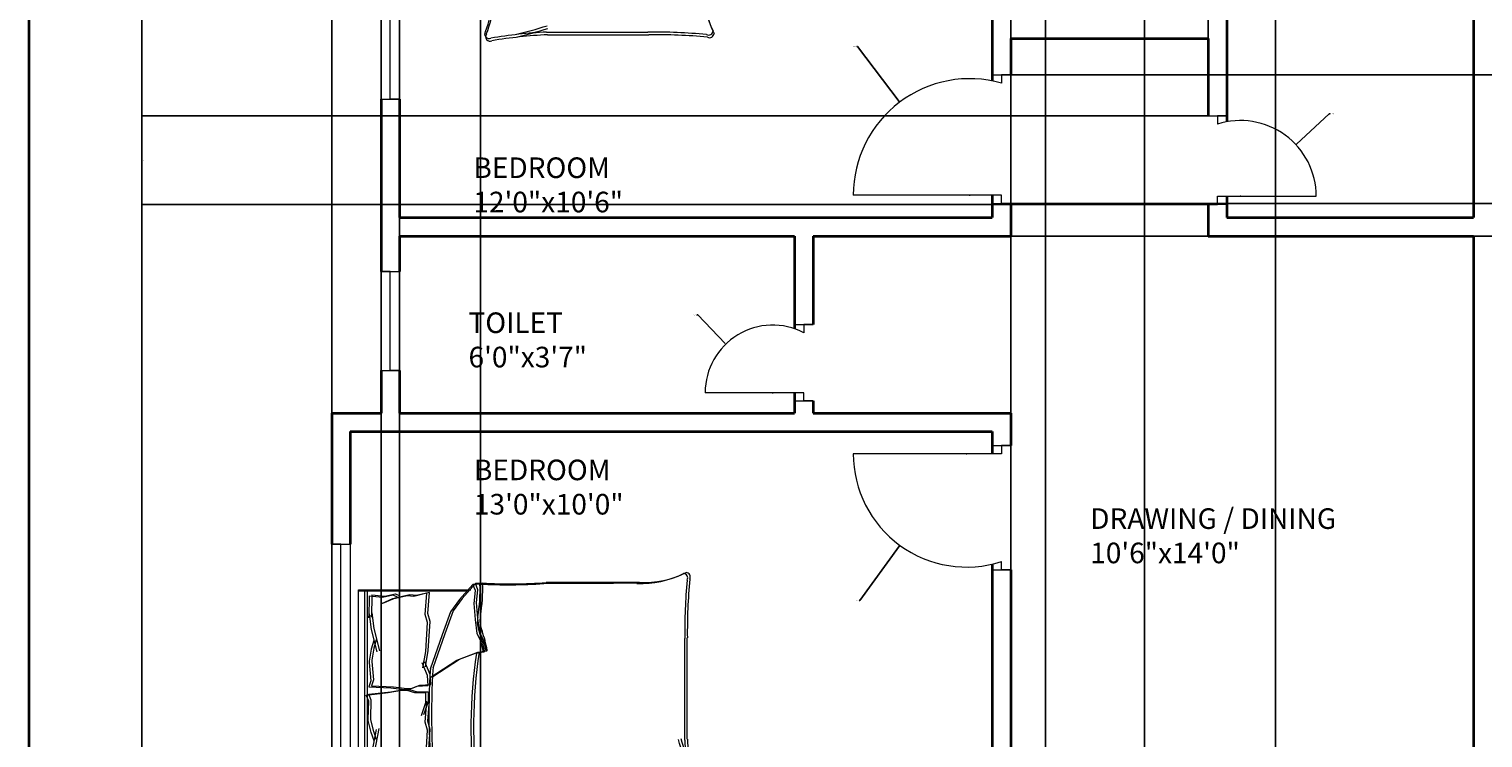
# Model space of a CAD drawing. Units: inches. Extents: x 1937 to 2996, y 1402 to 2323.
# Tile 5 of 10: x 1937 to 2290, y 1944 to 2116. Entities that reach past the tile are written whole.
import ezdxf

# ---------------------------------------------------------------- set-up
doc = ezdxf.new("R2010")
doc.units = ezdxf.units.IN
for name, color, linetype, lineweight in [('A-ANNO-DIMS', 2, 'Continuous', 18), ('A-ANNO-TTLB', 7, 'Continuous', 35), ('A-AREA-IDEN', 7, 'Continuous', 18), ('A-DOOR', 11, 'Continuous', 18), ('A-FURN', 8, 'Continuous', 13), ('A-GLAZ', 141, 'Continuous', 18), ('A-WALL', 7, 'Continuous', 35)]:
    doc.layers.add(name, color=color, linetype=linetype, lineweight=lineweight)
doc.styles.get("Standard").update_dxf_attribs({"font": 'arial.ttf'})
doc.dimstyles.get("Standard").update_dxf_attribs({"dimtxt": 0.18, "dimasz": 0.18, "dimexe": 0.18, "dimexo": 0.0625, "dimgap": 0.09, "dimtad": 0, "dimtih": 1, "dimtoh": 1, "dimdec": 4, "dimzin": 0, "dimdsep": 46, "dimtxsty": 'Standard', "dimcen": 0.09, "dimadec": 0, "dimazin": 0, "dimtfac": 1, "dimtdec": 4, "dimtofl": 0, "dimtmove": 0, "dimatfit": 3, "dimfxl": 1, "dimtolj": 1, "dimtzin": 0, "dimarcsym": 0})

# ---------------------------------------------------------------- blocks, each defined once
blk = doc.blocks.new('BED-DOUBLE')
for p, q in [((-24.01, -18.11), (-24.01, 0)), ((-24.01, -18.11), (-24.01, 0)), ((-24.01, 0), (24.01, 0)), ((23.78, 0), (23.78, -26.61)), ((23.78, 0), (23.78, -26.61)), ((24.01, 0), (24.01, -0.64)), ((-24.01, -1.53), (23.78, -1.53)), ((-24.01, -1.53), (23.78, -1.53)), ((-23.78, -18.75), (-23.78, -0.64)), ((-23.78, -18.75), (-23.78, -0.64)), ((-23.78, -2.17), (24.01, -2.17)), ((-23.78, -2.17), (24.01, -2.17)), ((-23.59, -3.34), (-19.3, -3.01)), ((-23.59, -3.34), (-19.31, -3.01)), ((-23.59, -3.32), (-23.01, -6.5)), ((-23.59, -3.32), (-23.01, -6.5)), ((-19.31, -3.01), (-19.2, -3.03)), ((-19.3, -3.01), (-19.2, -3.03)), ((-19.2, -3.03), (-15.38, -3.32)), ((-19.2, -3.03), (-15.38, -3.32)), ((-15.38, -3.32), (-9.88, -4.33)), ((-15.38, -3.32), (-9.88, -4.33)), ((-12.63, -3.75), (-10.61, -3.03)), ((-12.63, -3.75), (-10.61, -3.03)), ((-10.61, -3.03), (-7.71, -2.3)), ((-10.61, -3.03), (-7.71, -2.3)), ((-10.38, -3.67), (-7.49, -2.94)), ((-10.38, -3.67), (-7.49, -2.94)), ((-7.71, -2.3), (-7.39, -2.3)), ((-7.71, -2.3), (-7.39, -2.3)), ((-7.49, -2.94), (-7.16, -2.94)), ((-7.49, -2.94), (-7.16, -2.94)), ((-7.39, -2.3), (-2.95, -2.45)), ((-7.39, -2.3), (-2.95, -2.45)), ((-7.16, -2.94), (-2.72, -3.09)), ((-7.16, -2.94), (-2.72, -3.09)), ((-2.95, -2.45), (-1.5, -1.87)), ((-2.95, -2.45), (-1.5, -1.87)), ((-2.72, -3.09), (-1.27, -2.51)), ((-2.72, -3.09), (-1.27, -2.51)), ((-1.5, -1.87), (-0.92, -7.22)), ((-1.5, -1.87), (-0.92, -7.22)), ((-1.27, -2.51), (-0.7, -7.86)), ((-1.27, -2.51), (-0.7, -7.86)), ((0.49, -2.49), (0.25, -7.87)), ((0.49, -2.49), (0.25, -7.87)), ((0.72, -3.13), (0.48, -8.51)), ((0.72, -3.13), (0.48, -8.51)), ((1.97, -2.98), (0.49, -2.49)), ((1.97, -2.98), (0.49, -2.49)), ((2.2, -3.62), (0.72, -3.13)), ((2.2, -3.62), (0.72, -3.13)), ((6.4, -2.56), (1.97, -2.98)), ((6.4, -2.56), (1.97, -2.98)), ((6.63, -3.2), (2.2, -3.62)), ((6.63, -3.2), (2.2, -3.62)), ((6.72, -2.54), (6.4, -2.56)), ((6.72, -2.54), (6.4, -2.56)), ((6.95, -3.18), (6.63, -3.2)), ((6.95, -3.18), (6.63, -3.2)), ((9.65, -3.08), (6.72, -2.54)), ((9.65, -3.08), (6.72, -2.54)), ((9.88, -3.72), (6.95, -3.18)), ((9.88, -3.72), (6.95, -3.18)), ((14.43, -3.07), (9.01, -4.42)), ((14.43, -3.07), (9.01, -4.42)), ((11.72, -3.67), (9.65, -3.08)), ((11.72, -3.67), (9.65, -3.08)), ((18.23, -2.54), (14.43, -3.07)), ((18.23, -2.54), (14.43, -3.07)), ((18.46, -3.18), (14.66, -3.71)), ((18.46, -3.18), (14.66, -3.71)), ((22.63, -2.56), (17.23, -2.46)), ((17.23, -2.46), (18.23, -2.54)), ((22.63, -2.56), (17.23, -2.46)), ((17.23, -2.46), (18.23, -2.54)), ((22.86, -3.2), (17.45, -3.1)), ((17.45, -3.1), (18.46, -3.18)), ((22.86, -3.2), (17.45, -3.1)), ((17.45, -3.1), (18.46, -3.18)), ((22.63, -2.56), (22.25, -5.77)), ((22.63, -2.56), (22.25, -5.77)), ((22.86, -3.2), (22.48, -6.41)), ((22.86, -3.2), (22.48, -6.41)), ((24.01, -0.64), (24.01, -27.25)), ((24.01, -0.64), (24.01, -27.25)), ((-23.01, -6.5), (-23.45, -9.1)), ((-23.01, -6.5), (-23.45, -9.1)), ((-23.36, -3.98), (-19.08, -3.65)), ((-23.36, -3.98), (-19.08, -3.65)), ((-23.36, -3.96), (-22.78, -7.14)), ((-23.36, -3.96), (-22.78, -7.14)), ((-22.43, -8.96), (-21.42, -6.21)), ((-22.43, -8.96), (-21.42, -6.21)), ((-22.21, -9.59), (-21.19, -6.85)), ((-22.2, -9.59), (-21.19, -6.85)), ((-19.08, -3.65), (-18.97, -3.67)), ((-19.08, -3.65), (-18.97, -3.67)), ((-18.97, -3.67), (-15.15, -3.96)), ((-18.97, -3.67), (-15.15, -3.96)), ((-15.15, -3.96), (-9.65, -4.97)), ((-15.15, -3.96), (-9.65, -4.97)), ((-12.4, -4.39), (-10.38, -3.67)), ((-12.4, -4.39), (-10.38, -3.67)), ((14.66, -3.71), (9.24, -5.06)), ((14.66, -3.71), (9.24, -5.06)), ((11.94, -4.31), (9.88, -3.72)), ((11.94, -4.31), (9.88, -3.72)), ((21.83, -8.26), (20.64, -5.58)), ((21.82, -8.26), (20.64, -5.58)), ((22.05, -8.9), (20.87, -6.22)), ((22.05, -8.9), (20.87, -6.22)), ((22.25, -5.77), (22.84, -8.34)), ((22.25, -5.77), (22.84, -8.34)), ((22.48, -6.41), (23.07, -8.98)), ((22.48, -6.41), (23.07, -8.98)), ((-23.45, -9.1), (-22.87, -10.11)), ((-23.45, -9.1), (-22.87, -10.11)), ((-22.78, -7.14), (-23.22, -9.74)), ((-22.78, -7.14), (-23.22, -9.74)), ((-23.22, -9.74), (-22.64, -10.75)), ((-23.22, -9.74), (-22.64, -10.75)), ((-23.01, -12.57), (-22.43, -8.96)), ((-23.01, -12.57), (-22.43, -8.96)), ((-22.78, -13.21), (-22.2, -9.59)), ((-22.78, -13.21), (-22.21, -9.59)), ((-0.92, -7.22), (-0.35, -10.4)), ((-0.92, -7.22), (-0.35, -10.4)), ((-0.7, -7.86), (-0.12, -11.04)), ((-0.7, -7.86), (-0.12, -11.04)), ((-0.35, -10.4), (-0.35, -11.7)), ((-0.35, -10.4), (-0.35, -11.7)), ((0.25, -7.87), (-0.13, -11.08)), ((0.25, -7.87), (-0.13, -11.08)), ((0.48, -8.51), (0.1, -11.72)), ((0.48, -8.51), (0.1, -11.72)), ((22.63, -11.83), (21.82, -8.26)), ((22.63, -11.83), (21.83, -8.26)), ((22.86, -12.47), (22.05, -8.9)), ((22.86, -12.47), (22.05, -8.9)), ((22.84, -8.34), (22.33, -9.38)), ((22.84, -8.34), (22.33, -9.38)), ((23.07, -8.98), (22.56, -10.02)), ((23.07, -8.98), (22.56, -10.02)), ((-22.72, -14.16), (-23.01, -12.57)), ((-22.72, -14.16), (-23.01, -12.57)), ((-22.49, -14.8), (-22.78, -13.21)), ((-22.49, -14.8), (-22.78, -13.21)), ((-0.35, -11.7), (-0.92, -13.58)), ((-0.35, -11.7), (-0.92, -13.58)), ((-0.92, -13.58), (-0.92, -16.26)), ((-0.92, -13.58), (-0.92, -16.26)), ((-0.12, -12.34), (-0.7, -14.22)), ((-0.12, -12.34), (-0.7, -14.22)), ((-0.13, -11.08), (-0.05, -12.38)), ((-0.13, -11.08), (-0.05, -12.38)), ((-0.12, -11.04), (-0.12, -12.34)), ((-0.12, -11.04), (-0.12, -12.34)), ((-0.05, -12.38), (0.65, -14.22)), ((-0.05, -12.38), (0.65, -14.22)), ((0.1, -11.72), (0.18, -13.02)), ((0.1, -11.72), (0.18, -13.02)), ((0.18, -13.02), (0.87, -14.86)), ((0.18, -13.02), (0.87, -14.86)), ((22.44, -13.43), (22.63, -11.83)), ((22.44, -13.43), (22.63, -11.83)), ((23.21, -16.57), (22.44, -13.43)), ((23.21, -16.57), (22.44, -13.43)), ((22.67, -14.07), (22.86, -12.47)), ((22.67, -14.07), (22.86, -12.47)), ((23.44, -17.21), (22.67, -14.07)), ((23.44, -17.21), (22.67, -14.07)), ((-23.3, -17.34), (-22.72, -14.16)), ((-23.3, -17.34), (-22.72, -14.16)), ((-18.2, -16.62), (-23.3, -17.34)), ((-18.2, -16.62), (-23.3, -17.34)), ((-23.07, -17.98), (-22.49, -14.8)), ((-23.07, -17.98), (-22.49, -14.8)), ((-17.98, -17.26), (-23.07, -17.98)), ((-17.98, -17.26), (-23.07, -17.98)), ((-21.1, -15.63), (-17.07, -16.3)), ((-21.1, -15.63), (-17.07, -16.3)), ((-20.87, -16.27), (-16.84, -16.93)), ((-20.87, -16.27), (-16.84, -16.93)), ((-17.07, -16.3), (-18.2, -16.62)), ((-17.07, -16.3), (-18.2, -16.62)), ((-16.84, -16.93), (-17.98, -17.26)), ((-16.84, -16.93), (-17.98, -17.26)), ((-17.07, -16.3), (-10.06, -16.73)), ((-17.07, -16.3), (-10.06, -16.73)), ((-16.84, -16.93), (-9.83, -17.37)), ((-16.84, -16.93), (-9.83, -17.37)), ((-10.06, -16.73), (-8.1, -16.17)), ((-10.06, -16.73), (-8.1, -16.17)), ((-9.83, -17.37), (-7.87, -16.81)), ((-9.83, -17.37), (-7.87, -16.81)), ((-8.1, -16.17), (-2.97, -16.57)), ((-8.1, -16.17), (-2.97, -16.57)), ((-7.87, -16.81), (-2.74, -17.21)), ((-7.87, -16.81), (-2.74, -17.21)), ((-3.38, -16.26), (-6.53, -15.17)), ((-3.38, -16.26), (-6.53, -15.17)), ((-3.15, -16.9), (-6.3, -15.81)), ((-3.15, -16.9), (-6.3, -15.81)), ((-0.92, -16.26), (-3.38, -16.26)), ((-0.92, -16.26), (-3.38, -16.26)), ((-0.7, -16.9), (-3.15, -16.9)), ((-0.7, -16.9), (-3.15, -16.9)), ((-0.7, -14.22), (-0.7, -16.9)), ((-0.7, -14.22), (-0.7, -16.9)), ((0.65, -14.22), (0.81, -16.89)), ((0.65, -14.22), (0.81, -16.89)), ((0.81, -16.89), (3.27, -16.74)), ((0.81, -16.89), (3.27, -16.74)), ((0.87, -14.86), (1.04, -17.53)), ((0.87, -14.86), (1.04, -17.53)), ((1.04, -17.53), (3.49, -17.38)), ((1.04, -17.53), (3.49, -17.38)), ((2.77, -17.38), (6.97, -23.88)), ((2.77, -17.38), (6.96, -23.88)), ((3.27, -16.74), (6.34, -15.45)), ((3.27, -16.74), (6.34, -15.45)), ((3.49, -17.38), (6.56, -16.09)), ((3.49, -17.38), (6.56, -16.09)), ((13.16, -20.32), (4.82, -17.38)), ((13.16, -20.32), (4.82, -17.38)), ((5.08, -15.63), (9.11, -16.3)), ((5.08, -15.63), (9.11, -16.3)), ((5.31, -16.27), (9.34, -16.93)), ((5.31, -16.27), (9.34, -16.93)), ((9.11, -16.3), (16.12, -16.73)), ((9.11, -16.3), (16.12, -16.73)), ((9.34, -16.93), (16.35, -17.37)), ((9.34, -16.93), (16.35, -17.37)), ((16.12, -16.73), (18.08, -16.17)), ((16.12, -16.73), (18.08, -16.17)), ((16.35, -17.37), (18.31, -16.81)), ((16.35, -17.37), (18.31, -16.81)), ((18.08, -16.17), (23.21, -16.57)), ((18.08, -16.17), (23.21, -16.57)), ((18.31, -16.81), (23.44, -17.21)), ((18.31, -16.81), (23.44, -17.21)), ((3, -18.02), (7.19, -24.52)), ((3, -18.02), (7.19, -24.52)), ((13.39, -20.96), (5.05, -18.02)), ((13.39, -20.96), (5.05, -18.02)), ((18.74, -22.33), (13.16, -20.32)), ((18.74, -22.33), (13.16, -20.32)), ((18.96, -22.97), (13.39, -20.96)), ((18.96, -22.97), (13.39, -20.96)), ((6.96, -23.88), (8.67, -28.37)), ((6.97, -23.88), (8.67, -28.37)), ((7.19, -24.52), (8.9, -29)), ((7.19, -24.52), (8.9, -29)), ((21.68, -24.5), (18.74, -22.33)), ((21.68, -24.5), (18.74, -22.33)), ((21.91, -25.13), (18.96, -22.97)), ((21.91, -25.13), (18.96, -22.97)), ((25.38, -27.75), (21.68, -24.5)), ((25.38, -27.75), (21.68, -24.5)), ((16.88, -28.37), (20.75, -28.06)), ((16.88, -28.37), (20.75, -28.06)), ((20.75, -28.06), (23.85, -28.37)), ((20.75, -28.06), (23.85, -28.37)), ((25.61, -28.39), (21.91, -25.13)), ((25.61, -28.39), (21.91, -25.13)), ((23.85, -28.37), (25.38, -27.75)), ((23.85, -28.37), (25.38, -27.75)), ((25.46, -29.49), (25.38, -27.75, 3.87)), ((25.46, -29.49), (25.38, -27.75, 3.87)), ((8.67, -28.37), (8.98, -30.38)), ((8.67, -28.37), (8.98, -30.38)), ((8.9, -29), (9.21, -31.02)), ((8.9, -29), (9.21, -31.02)), ((8.98, -30.38), (11.46, -29.76)), ((8.98, -30.38), (11.46, -29.76)), ((9.21, -31.02), (11.68, -30.4)), ((9.21, -31.02), (11.68, -30.4)), ((11.46, -29.76), (13.47, -28.83)), ((11.46, -29.76), (13.47, -28.83)), ((11.68, -30.4), (13.7, -29.47)), ((11.68, -30.4), (13.7, -29.47)), ((13.47, -28.83), (16.88, -28.37)), ((13.47, -28.83), (16.88, -28.37)), ((13.7, -29.47), (17.11, -29)), ((13.7, -29.47), (17.1, -29)), ((17.1, -29), (20.98, -28.69)), ((17.11, -29), (20.98, -28.69)), ((20.98, -28.69), (24.07, -29)), ((20.98, -28.69), (24.07, -29)), ((24.07, -29), (25.61, -28.39)), ((24.07, -29), (25.61, -28.39)), ((25.69, -30.13), (25.61, -28.39, 3.87)), ((25.69, -30.13), (25.61, -28.39, 3.87)), ((-12.42, -79.25), (12.19, -79.25)), ((-12.42, -79.25), (12.19, -79.25)), ((-12.19, -79.88), (12.42, -79.88)), ((-12.19, -79.88), (12.42, -79.88))]:
    blk.add_line(p, q)
for centre, radius, start, end in [((-6.13, -182.05), 164.97, 86.0865, 96.7821), ((-6.13, -182.05), 164.97, 86.0865, 96.7821), ((57.68, -20.1), 83.31, 178.7218, 185.604), ((57.68, -20.1), 83.31, 178.7218, 185.604), ((57.91, -20.74), 83.31, 178.7218, 185.604), ((57.91, -20.74), 83.31, 178.7218, 185.604), ((-5.9, -182.69), 164.97, 86.0865, 96.7821), ((-5.9, -182.69), 164.97, 86.0865, 96.7821), ((-9.73, -156.32), 129.02, 81.7845, 96.9006), ((-9.73, -156.32), 129.02, 81.7845, 96.9006), ((-9.5, -156.96), 129.02, 81.7845, 96.9006), ((-9.5, -156.96), 129.02, 81.7845, 96.9006), ((-194.79, -31.17), 170.11, 358.4762, 1.0082), ((-194.79, -31.17), 170.11, 358.4762, 1.0082), ((-194.56, -31.81), 170.11, 358.4762, 1.0082), ((-194.56, -31.81), 170.11, 358.4762, 1.0082), ((9.15, -30.44), 0.185, 160.2464, 271.1377), ((9.15, -30.44), 0.185, 160.2464, 271.1377), ((3.67, -1.48), 29.65, 280.6617, 289.8806), ((3.67, -1.48), 29.65, 280.6617, 289.8806), ((9.38, -31.08), 0.185, 160.2464, 271.1377), ((9.38, -31.08), 0.185, 160.2464, 271.1377), ((3.9, -2.12), 29.65, 280.6617, 289.8806), ((3.9, -2.12), 29.65, 280.6617, 289.8806), ((16.26, -35.07), 6.22, 78.6608, 113.7384), ((16.26, -35.07), 6.22, 78.6608, 113.7384), ((16.49, -35.71), 6.22, 78.6608, 113.7384), ((16.49, -35.71), 6.22, 78.6608, 113.7384), ((23.84, 6.66), 36.18, 259.8763, 272.5657), ((23.84, 6.66), 36.18, 259.8763, 272.5657), ((24.07, 6.02), 36.18, 259.8763, 272.5657), ((24.07, 6.02), 36.18, 259.8763, 272.5657), ((154.78, -36.32), 129.5, 176.9791, 183.8365), ((154.78, -36.32), 129.5, 176.9791, 183.8365), ((155.01, -36.95), 129.5, 176.9791, 183.8365), ((155.01, -36.95), 129.5, 176.9791, 183.8365), ((457.34, -50.61), 482.31, 178.2277, 181.7185), ((457.34, -50.61), 482.31, 178.2277, 181.7185), ((457.57, -51.25), 482.31, 178.2277, 181.7185), ((457.57, -51.25), 482.31, 178.2277, 181.7185), ((-4536.23, -67.82), 4561.86, 0.00217, 0.28689), ((-4536.23, -67.82), 4561.86, 0.00217, 0.28689), ((-4536, -68.46), 4561.86, 0.00217, 0.28689), ((-4536, -68.46), 4561.86, 0.00217, 0.28689), ((-54.38, -64.52), 29.63, 346.0648, 358.9113), ((-54.38, -64.52), 29.63, 346.0648, 358.9113), ((-54.16, -65.15), 29.63, 346.0648, 358.9113), ((-54.16, -65.15), 29.63, 346.0648, 358.9113), ((48.67, -68.67), 23.07, 177.4714, 206.4681), ((48.67, -68.67), 23.07, 177.4714, 206.4681), ((48.9, -69.31), 23.07, 177.4714, 206.4681), ((48.9, -69.31), 23.07, 177.4714, 206.4681), ((-49.14, -70.28), 23.56, 337.9751, 356.652), ((-49.14, -70.28), 23.56, 337.9751, 356.652), ((-48.92, -70.91), 23.56, 337.9751, 356.652), ((-48.92, -70.91), 23.56, 337.9751, 356.652), ((-44.71, 23.71), 106.46, 283.3832, 287.7053), ((-44.71, 23.71), 106.46, 283.3832, 287.7053), ((-26.4, -79.72), 1.09, 146.1736, 293.4781), ((-26.4, -79.72), 1.09, 146.1736, 293.4781), ((-26.17, -80.36), 1.09, 146.1736, 293.4781), ((-26.17, -80.36), 1.09, 146.1736, 293.4781), ((-6.06, -200.84), 121.76, 92.9958, 99.4091), ((-6.06, -200.84), 121.76, 92.9958, 99.4091), ((-5.83, -201.48), 121.76, 92.9958, 99.4091), ((-5.83, -201.48), 121.76, 92.9958, 99.4091), ((-44.48, 23.07), 106.46, 283.3832, 287.7053), ((-44.48, 23.07), 106.46, 283.3832, 287.7053), ((13.67, -212.28), 133.04, 84.4998, 90.6351), ((13.67, -212.28), 133.04, 84.4998, 90.6351), ((13.9, -212.92), 133.04, 84.4998, 90.6351), ((13.9, -212.92), 133.04, 84.4998, 90.6351), ((26.93, -78.87), 1.1, 242.6588, 356.02), ((26.93, -78.87), 1.1, 242.6588, 356.02), ((27.15, -79.51), 1.1, 242.6588, 356.02), ((27.15, -79.51), 1.1, 242.6588, 356.02)]:
    blk.add_arc(centre, radius, start, end)
blk = doc.blocks.new('WINDOW-60IN')
for p, q in [((0, 2.25), (0, -2.25)), ((0, 2.25), (60, 2.25)), ((0, -2.25), (0, 0)), ((0, 0), (60, 0)), ((60, 0), (60, 2.25)), ((60, 2.25), (60, -2.25)), ((60, -2.25), (0, -2.25))]:
    blk.add_line(p, q)
blk = doc.blocks.new('WINDOW-24IN')
for p, q in [((0, -2.25), (0, 2.25)), ((0, 2.25), (0, 0)), ((24, 2.25), (0, 2.25)), ((0, 0), (24, 0)), ((24, -2.25), (24, 2.25)), ((24, 0), (24, -2.25)), ((0, -2.25), (24, -2.25))]:
    blk.add_line(p, q)
blk = doc.blocks.new('*D24')
at = {"layer": 'A-ANNO-DIMS', "color": 0, "lineweight": -2, "transparency": 16777216}
for p, q in [((2022.58, 2236.81), (1964.32, 2236.81)), ((1964.5, 2236.63), (1964.5, 1896.24)), ((1964.5, 1555.49), (1964.5, 1895.87)), ((2022.58, 1555.31), (1964.32, 1555.31))]:
    blk.add_line(p, q, dxfattribs=at)
at = {"layer": 'A-ANNO-DIMS', "color": 0, "transparency": 16777216}
for points in [[(1964.47, 2236.63), (1964.53, 2236.63), (1964.5, 2236.81)], [(1964.47, 1555.49), (1964.53, 1555.49), (1964.5, 1555.31)]]:
    blk.add_solid(points, dxfattribs=at)
at = {"layer": 'Defpoints', "color": 0, "transparency": 16777216}
for p in [(1964.5, 2236.81), (2022.65, 2236.81), (2022.65, 1555.31)]:
    blk.add_point(p, dxfattribs=at)
at = {"layer": 'A-ANNO-DIMS', "color": 0, "transparency": 16777216, "insert": (1964.5, 1896.06), "char_height": 0.18, "attachment_point": 5}
blk.add_mtext('\\A1;681.5', dxfattribs=at)
blk = doc.blocks.new('*D44')
at = {"layer": 'A-ANNO-DIMS', "color": 0, "lineweight": -2, "transparency": 16777216}
for p, q in [((2010.65, 1769.37), (2010.65, 2283.14)), ((2010.83, 2282.96), (2016.44, 2282.96)), ((2022.47, 2282.96), (2016.86, 2282.96)), ((2022.65, 1769.37), (2022.65, 2283.14))]:
    blk.add_line(p, q, dxfattribs=at)
at = {"layer": 'A-ANNO-DIMS', "color": 0, "transparency": 16777216}
for points in [[(2010.83, 2282.99), (2010.83, 2282.93), (2010.65, 2282.96)], [(2022.47, 2282.99), (2022.47, 2282.93), (2022.65, 2282.96)]]:
    blk.add_solid(points, dxfattribs=at)
at = {"layer": 'Defpoints', "color": 0, "transparency": 16777216}
for p in [(2022.65, 2282.96), (2010.65, 1769.31), (2022.65, 1769.31)]:
    blk.add_point(p, dxfattribs=at)
at = {"layer": 'A-ANNO-DIMS', "color": 0, "transparency": 16777216, "insert": (2016.65, 2282.96), "char_height": 0.18, "attachment_point": 5}
blk.add_mtext('\\A1;12', dxfattribs=at)
blk = doc.blocks.new('*D46')
at = {"layer": 'A-ANNO-DIMS', "color": 0, "lineweight": -2, "transparency": 16777216}
for p, q in [((2027.15, 1591.37), (2027.15, 2283.14)), ((2027.33, 2282.96), (2036.53, 2282.96)), ((2046.64, 2282.96), (2037.44, 2282.96)), ((2046.82, 1591.37), (2046.82, 2283.14))]:
    blk.add_line(p, q, dxfattribs=at)
at = {"layer": 'A-ANNO-DIMS', "color": 0, "transparency": 16777216}
for points in [[(2027.33, 2282.99), (2027.33, 2282.93), (2027.15, 2282.96)], [(2046.64, 2282.99), (2046.64, 2282.93), (2046.82, 2282.96)]]:
    blk.add_solid(points, dxfattribs=at)
at = {"layer": 'Defpoints', "color": 0, "transparency": 16777216}
for p in [(2046.82, 2282.96), (2027.15, 1591.31), (2046.82, 1591.31)]:
    blk.add_point(p, dxfattribs=at)
at = {"layer": 'A-ANNO-DIMS', "color": 0, "transparency": 16777216, "insert": (2036.99, 2282.96), "char_height": 0.18, "attachment_point": 5}
blk.add_mtext('\\A1;19.678', dxfattribs=at)
blk = doc.blocks.new('*D47')
at = {"layer": 'A-ANNO-DIMS', "color": 0, "lineweight": -2, "transparency": 16777216}
for p, q in [((2175.65, 1591.37), (2175.65, 2283.14)), ((2175.83, 2282.96), (2179.52, 2282.96)), ((2183.96, 2282.96), (2180.27, 2282.96)), ((2184.14, 1591.37), (2184.14, 2283.14))]:
    blk.add_line(p, q, dxfattribs=at)
at = {"layer": 'A-ANNO-DIMS', "color": 0, "transparency": 16777216}
for points in [[(2175.83, 2282.99), (2175.83, 2282.93), (2175.65, 2282.96)], [(2183.96, 2282.99), (2183.96, 2282.93), (2184.14, 2282.96)]]:
    blk.add_solid(points, dxfattribs=at)
at = {"layer": 'Defpoints', "color": 0, "transparency": 16777216}
for p in [(2184.14, 2282.96), (2175.65, 1591.31), (2184.14, 1591.31)]:
    blk.add_point(p, dxfattribs=at)
at = {"layer": 'A-ANNO-DIMS', "color": 0, "transparency": 16777216, "insert": (2179.89, 2282.96), "char_height": 0.18, "attachment_point": 5}
blk.add_mtext('\\A1;8.491', dxfattribs=at)
blk = doc.blocks.new('*D48')
at = {"layer": 'A-ANNO-DIMS', "color": 0, "lineweight": -2, "transparency": 16777216}
for p, q in [((2208.14, 1591.37), (2208.14, 2283.14)), ((2208.32, 2282.96), (2223.66, 2282.96)), ((2239.78, 2282.96), (2224.44, 2282.96)), ((2239.96, 1591.37), (2239.96, 2283.14))]:
    blk.add_line(p, q, dxfattribs=at)
at = {"layer": 'A-ANNO-DIMS', "color": 0, "transparency": 16777216}
for points in [[(2208.32, 2282.99), (2208.32, 2282.93), (2208.14, 2282.96)], [(2239.78, 2282.99), (2239.78, 2282.93), (2239.96, 2282.96)]]:
    blk.add_solid(points, dxfattribs=at)
at = {"layer": 'Defpoints', "color": 0, "transparency": 16777216}
for p in [(2239.96, 2282.96), (2208.14, 1591.31), (2239.96, 1591.31)]:
    blk.add_point(p, dxfattribs=at)
at = {"layer": 'A-ANNO-DIMS', "color": 0, "transparency": 16777216, "insert": (2224.05, 2282.96), "char_height": 0.18, "attachment_point": 5}
blk.add_mtext('\\A1;31.82', dxfattribs=at)
blk = doc.blocks.new('*D49')
at = {"layer": 'A-ANNO-DIMS', "color": 0, "lineweight": -2, "transparency": 16777216}
for p, q in [((2223.65, 2095.03), (2223.65, 2283.14)), ((2223.83, 2282.96), (2225.64, 2282.96)), ((2227.97, 2282.96), (2226.16, 2282.96)), ((2228.15, 2095.03), (2228.15, 2283.14))]:
    blk.add_line(p, q, dxfattribs=at)
at = {"layer": 'A-ANNO-DIMS', "color": 0, "transparency": 16777216}
for points in [[(2223.83, 2282.99), (2223.83, 2282.93), (2223.65, 2282.96)], [(2227.97, 2282.99), (2227.97, 2282.93), (2228.15, 2282.96)]]:
    blk.add_solid(points, dxfattribs=at)
at = {"layer": 'Defpoints', "color": 0, "transparency": 16777216}
for p in [(2228.15, 2282.96), (2223.65, 2094.97), (2228.15, 2094.97)]:
    blk.add_point(p, dxfattribs=at)
at = {"layer": 'A-ANNO-DIMS', "color": 0, "transparency": 16777216, "insert": (2225.9, 2282.96), "char_height": 0.18, "attachment_point": 5}
blk.add_mtext('\\A1;4.5', dxfattribs=at)
blk = doc.blocks.new('*D51')
at = {"layer": 'A-ANNO-DIMS', "color": 0, "lineweight": -2, "transparency": 16777216}
for p, q in [((2175.71, 2073.74), (2970.48, 2073.74)), ((2970.3, 2073.56), (2970.3, 2069.95)), ((2970.3, 2065.99), (2970.3, 2069.59)), ((2175.71, 2065.81), (2970.48, 2065.81))]:
    blk.add_line(p, q, dxfattribs=at)
at = {"layer": 'A-ANNO-DIMS', "color": 0, "transparency": 16777216}
for points in [[(2970.27, 2073.56), (2970.33, 2073.56), (2970.3, 2073.74)], [(2970.27, 2065.99), (2970.33, 2065.99), (2970.3, 2065.81)]]:
    blk.add_solid(points, dxfattribs=at)
at = {"layer": 'Defpoints', "color": 0, "transparency": 16777216}
for p in [(2175.65, 2073.74), (2970.3, 2073.74), (2175.65, 2065.81)]:
    blk.add_point(p, dxfattribs=at)
at = {"layer": 'A-ANNO-DIMS', "color": 0, "transparency": 16777216, "insert": (2970.3, 2069.77), "char_height": 0.18, "attachment_point": 5}
blk.add_mtext('\\A1;7.931', dxfattribs=at)
blk = doc.blocks.new('*D52')
at = {"layer": 'A-ANNO-DIMS', "color": 0, "lineweight": -2, "transparency": 16777216}
for p, q in [((2175.71, 2104.94), (2970.48, 2104.94)), ((2970.3, 2104.76), (2970.3, 2089.52)), ((2970.3, 2073.92), (2970.3, 2089.16)), ((2175.71, 2073.74), (2970.48, 2073.74))]:
    blk.add_line(p, q, dxfattribs=at)
at = {"layer": 'A-ANNO-DIMS', "color": 0, "transparency": 16777216}
for points in [[(2970.27, 2104.76), (2970.33, 2104.76), (2970.3, 2104.94)], [(2970.27, 2073.92), (2970.33, 2073.92), (2970.3, 2073.74)]]:
    blk.add_solid(points, dxfattribs=at)
at = {"layer": 'Defpoints', "color": 0, "transparency": 16777216}
for p in [(2175.65, 2104.94), (2970.3, 2104.94), (2175.65, 2073.74)]:
    blk.add_point(p, dxfattribs=at)
at = {"layer": 'A-ANNO-DIMS', "color": 0, "transparency": 16777216, "insert": (2970.3, 2089.34), "char_height": 0.18, "attachment_point": 5}
blk.add_mtext('\\A1;31.204', dxfattribs=at)
blk = doc.blocks.new('*D54')
at = {"layer": 'A-ANNO-DIMS', "color": 0, "lineweight": -2, "transparency": 16777216}
for p, q in [((2223.58, 2094.97), (1964.32, 2094.97)), ((1964.5, 2094.79), (1964.5, 2084.39)), ((1964.5, 2073.63), (1964.5, 2084.03)), ((2223.58, 2073.45), (1964.32, 2073.45))]:
    blk.add_line(p, q, dxfattribs=at)
at = {"layer": 'A-ANNO-DIMS', "color": 0, "transparency": 16777216}
for points in [[(1964.47, 2094.79), (1964.53, 2094.79), (1964.5, 2094.97)], [(1964.47, 2073.63), (1964.53, 2073.63), (1964.5, 2073.45)]]:
    blk.add_solid(points, dxfattribs=at)
at = {"layer": 'Defpoints', "color": 0, "transparency": 16777216}
for p in [(1964.5, 2094.97), (2223.65, 2094.97), (2223.65, 2073.45)]:
    blk.add_point(p, dxfattribs=at)
at = {"layer": 'A-ANNO-DIMS', "color": 0, "transparency": 16777216, "insert": (1964.5, 2084.21), "char_height": 0.18, "attachment_point": 5}
blk.add_mtext('\\A1;21.518', dxfattribs=at)
blk = doc.blocks.new('*D66')
at = {"layer": 'A-ANNO-DIMS', "color": 0, "lineweight": -2, "transparency": 16777216}
for p, q in [((2138.22, 2111.84), (2138.4, 2111.84)), ((2138.4, 2111.84), (2148.52, 2098.44)), ((2165.59, 2075.74), (2165.77, 2075.74)), ((2165.68, 2075.65), (2165.68, 2075.83))]:
    blk.add_line(p, q, dxfattribs=at)
at = {"layer": 'A-ANNO-DIMS', "color": 0, "transparency": 16777216}
blk.add_solid([(2148.54, 2098.46), (2148.49, 2098.42), (2148.63, 2098.3)], dxfattribs=at)
at = {"layer": 'Defpoints', "color": 0, "transparency": 16777216}
for p in [(2148.63, 2098.3), (2165.68, 2075.74)]:
    blk.add_point(p, dxfattribs=at)
at = {"layer": 'A-ANNO-DIMS', "color": 0, "transparency": 16777216, "insert": (2137.74, 2111.84), "char_height": 0.18, "attachment_point": 5}
blk.add_mtext('\\A1;R28.28', dxfattribs=at)
blk = doc.blocks.new('*D68')
at = {"layer": 'A-ANNO-DIMS', "color": 0, "lineweight": -2, "transparency": 16777216}
for p, q in [((2164.84, 2012.95), (2165.02, 2012.95)), ((2164.93, 2012.86), (2164.93, 2013.04)), ((2139.01, 1977.33), (2148.62, 1990.55)), ((2138.83, 1977.33), (2139.01, 1977.33))]:
    blk.add_line(p, q, dxfattribs=at)
at = {"layer": 'A-ANNO-DIMS', "color": 0, "transparency": 16777216}
blk.add_solid([(2148.6, 1990.56), (2148.65, 1990.53), (2148.73, 1990.69)], dxfattribs=at)
at = {"layer": 'Defpoints', "color": 0, "transparency": 16777216}
for p in [(2164.93, 2012.95), (2148.73, 1990.69)]:
    blk.add_point(p, dxfattribs=at)
at = {"layer": 'A-ANNO-DIMS', "color": 0, "transparency": 16777216, "insert": (2138.35, 1977.33), "char_height": 0.18, "attachment_point": 5}
blk.add_mtext('\\A1;R27.53', dxfattribs=at)
blk = doc.blocks.new('*D74')
at = {"layer": 'A-ANNO-DIMS', "color": 0, "lineweight": -2, "transparency": 16777216}
for p, q in [((2253.06, 2095.49), (2245.11, 2088.1)), ((2253.24, 2095.49), (2253.06, 2095.49)), ((2231.41, 2075.45), (2231.59, 2075.45)), ((2231.5, 2075.36), (2231.5, 2075.54))]:
    blk.add_line(p, q, dxfattribs=at)
at = {"layer": 'A-ANNO-DIMS', "color": 0, "transparency": 16777216}
blk.add_solid([(2245.09, 2088.12), (2245.13, 2088.08), (2244.97, 2087.98)], dxfattribs=at)
at = {"layer": 'Defpoints', "color": 0, "transparency": 16777216}
for p in [(2244.97, 2087.98), (2231.5, 2075.45)]:
    blk.add_point(p, dxfattribs=at)
at = {"layer": 'A-ANNO-DIMS', "color": 0, "transparency": 16777216, "insert": (2253.79, 2095.49), "char_height": 0.18, "attachment_point": 5}
blk.add_mtext('\\A1;R18.393', dxfattribs=at)
blk = doc.blocks.new('*D75')
at = {"layer": 'A-ANNO-DIMS', "color": 0, "lineweight": -2, "transparency": 16777216}
for p, q in [((2099.4, 2046.66), (2099.58, 2046.66)), ((2099.58, 2046.66), (2106.29, 2039.7)), ((2117.72, 2027.76), (2117.9, 2027.76)), ((2117.81, 2027.67), (2117.81, 2027.85))]:
    blk.add_line(p, q, dxfattribs=at)
at = {"layer": 'A-ANNO-DIMS', "color": 0, "transparency": 16777216}
blk.add_solid([(2106.31, 2039.72), (2106.27, 2039.68), (2106.42, 2039.57)], dxfattribs=at)
at = {"layer": 'Defpoints', "color": 0, "transparency": 16777216}
for p in [(2106.42, 2039.57), (2117.81, 2027.76)]:
    blk.add_point(p, dxfattribs=at)
at = {"layer": 'A-ANNO-DIMS', "color": 0, "transparency": 16777216, "insert": (2098.94, 2046.66), "char_height": 0.18, "attachment_point": 5}
blk.add_mtext('\\A1;R16.41', dxfattribs=at)

msp = doc.modelspace()

# ---------------------------------------------------------------- linework, layer by layer
at = {"layer": 'A-ANNO-TTLB'}
msp.add_lwpolyline([(1937.1125, 2323.2883), (2995.8132, 2323.2883), (2995.8132, 1401.6335), (1937.1125, 1401.6335)], close=True, dxfattribs=at)
at = {"layer": 'A-DOOR'}
for p, q in [((2171.1473, 2104.9416), (2175.6473, 2104.9416)), ((2175.6473, 2104.9416), (2173.3973, 2104.9416)), ((2173.3973, 2104.9416), (2173.3973, 2102.9416)), ((2223.6473, 2094.9699), (2228.1473, 2094.9699)), ((2228.1473, 2094.9699), (2225.8973, 2094.9699)), ((2225.8973, 2094.9699), (2225.8973, 2092.9699)), ((2173.3973, 2075.7376), (2137.3973, 2075.7376)), ((2173.3973, 2073.7376), (2173.3973, 2075.7376)), ((2225.8973, 2073.4521), (2225.8973, 2075.4521)), ((2225.8973, 2075.4521), (2249.8973, 2075.4521)), ((2171.1473, 2073.7376), (2175.6473, 2073.7376)), ((2175.6473, 2073.7376), (2173.3973, 2073.7376)), ((2228.1473, 2073.4521), (2223.6473, 2073.4521)), ((2223.6473, 2073.4521), (2225.8973, 2073.4521)), ((2123.1473, 2044.3061), (2127.6473, 2044.3061)), ((2127.6473, 2044.3061), (2125.3973, 2044.3061)), ((2125.3973, 2044.3061), (2125.3973, 2042.3061)), ((2125.3973, 2027.7551), (2101.3973, 2027.7551)), ((2123.1473, 2025.7551), (2127.6473, 2025.7551)), ((2125.3973, 2025.7551), (2125.3973, 2027.7551)), ((2127.6473, 2025.7551), (2125.3973, 2025.7551)), ((2171.1473, 2014.9523), (2175.6473, 2014.9523)), ((2175.6473, 2014.9523), (2173.3973, 2014.9523)), ((2173.3973, 2014.9523), (2173.3973, 2012.9523)), ((2173.3973, 2012.9523), (2137.3973, 2012.9523)), ((2173.3973, 1984.7551), (2173.3973, 1986.7551)), ((2171.1473, 1984.7551), (2175.6473, 1984.7551)), ((2175.6473, 1984.7551), (2173.3973, 1984.7551))]:
    msp.add_line(p, q, dxfattribs=at)
for centre, radius, start, end in [((2165.6759, 2075.7376), 28.2786, 74.154207, 180), ((2231.5041, 2075.4521), 18.3932, 360, 107.747927), ((2117.8084, 2027.7551), 16.4111, 62.456091, 180), ((2164.9292, 2012.9523), 27.5318, 180, 287.913245)]:
    msp.add_arc(centre, radius, start, end, dxfattribs=at)
at = {"layer": 'A-WALL'}
for p, q in [((2228.1473, 2196.3061), (2228.1473, 2093.5364)), ((2288.1473, 2196.3061), (2288.1473, 2070.3061)), ((2171.1473, 2121.8495), (2171.1473, 2103.4818)), ((2175.6473, 2113.8061), (2223.6473, 2113.8061)), ((2175.6473, 2113.8061), (2175.6473, 2104.9416)), ((2223.6473, 2113.8061), (2223.6473, 2094.9699)), ((2022.6473, 2099.0049), (2022.6473, 2057.1802)), ((2027.1473, 2099.0049), (2027.1473, 2070.3061)), ((2171.1473, 2075.7376), (2171.1473, 2070.3061)), ((2228.1473, 2075.4521), (2228.1473, 2070.3061)), ((2027.1473, 2070.3061), (2171.1473, 2070.3061)), ((2175.6473, 2073.7376), (2175.6473, 2065.8061)), ((2223.6473, 2073.4521), (2223.6473, 2065.8061)), ((2228.1473, 2070.3061), (2288.1473, 2070.3061)), ((2027.1473, 2065.8061), (2123.1473, 2065.8061)), ((2027.1473, 2065.8061), (2027.1473, 2057.1802)), ((2123.1473, 2065.8061), (2123.1473, 2043.2735)), ((2127.6473, 2065.8061), (2127.6473, 2044.3061)), ((2127.6473, 2065.8061), (2175.6473, 2065.8061)), ((2223.6473, 2065.8061), (2288.1473, 2065.8061)), ((2288.1473, 2065.8061), (2288.1473, 1932.2265)), ((2022.6473, 2033.1802), (2022.6473, 2022.8061)), ((2027.1473, 2033.1802), (2027.1473, 2022.8061)), ((2123.1473, 2027.7551), (2123.1473, 2022.8061)), ((2127.6473, 2025.7551), (2127.6473, 2022.8061)), ((2010.6473, 2022.8061), (2022.6473, 2022.8061)), ((2010.6473, 2022.8061), (2010.6473, 1990.9695)), ((2027.1473, 2022.8061), (2123.1473, 2022.8061)), ((2127.6473, 2022.8061), (2175.6473, 2022.8061)), ((2175.6473, 2022.8061), (2175.6473, 2014.9523)), ((2015.1473, 2018.3061), (2171.1473, 2018.3061)), ((2015.1473, 2018.3061), (2015.1473, 1990.9695)), ((2171.1473, 2018.3061), (2171.1473, 2012.9523)), ((2171.1473, 1986.1318), (2171.1473, 1898.3061)), ((2175.6473, 1984.7551), (2175.6473, 1898.3061))]:
    msp.add_line(p, q, dxfattribs=at)

# ---------------------------------------------------------------- block references
at = {"layer": 'A-FURN'}
msp.add_blockref('BED-DOUBLE', (2075.3048, 2194.5807), dxfattribs=at)
at = {"layer": 'A-FURN', "rotation": 89.99999983318573}
msp.add_blockref('BED-DOUBLE', (2017.1846, 1955.8397), dxfattribs=at)
at = {"layer": 'A-GLAZ', "rotation": 90}
for p in [(2024.8973, 2099.0049), (2012.8973, 1930.9695)]:
    msp.add_blockref('WINDOW-60IN', p, dxfattribs=at)
at = {"layer": 'A-GLAZ', "extrusion": (0, 0, -1), "zscale": -1, "rotation": 90}
msp.add_blockref('WINDOW-24IN', (-2024.8973, 2033.1802), dxfattribs=at)

# ---------------------------------------------------------------- texts
at = {"layer": 'A-AREA-IDEN', "char_height": 5, "attachment_point": 1}
for s, width, insert in [('BEDROOM\\P12\'0"x10\'6"', 267.145668, (2045.0806, 2084.8942)), ('TOILET\\P6\'0"x3\'7"', 102.162825, (2043.8932, 2047.248)), ('BEDROOM\\P13\'0"x10\'0"', 189.008899, (2045.2134, 2011.5102)), ('DRAWING / DINING \\P10\'6"x14\'0"', 244.68877, (2194.9624, 1999.6807))]:
    msp.add_mtext_dynamic_manual_height_columns(s, width=width, gutter_width=12.5, heights=[0], dxfattribs=dict(at, insert=insert))

# ---------------------------------------------------------------- dimensions: what is measured, and where the dimension line sits
at = {"layer": 'A-ANNO-DIMS'}
for base, p1, p2, override, picture, middle in [((2022.6473, 2282.9561), (2010.6473, 1769.3061), (2022.6473, 1769.3061), {"dimdec": 0, "dimlfac": 1, "dimrnd": 0, "dimzin": 0, "dimdsep": 46, "dimlunit": 2}, '*D44', (2016.6473, 2282.9561)), ((2046.82483, 2282.95612), (2027.14731, 1591.30612), (2046.82483, 1591.30612), {"dimdec": 3, "dimlfac": 1, "dimrnd": 0, "dimzin": 0, "dimdsep": 46, "dimlunit": 2}, '*D46', (2036.98607, 2282.95612)), ((2184.1385, 2282.9561), (2175.6473, 1591.3061), (2184.1385, 1591.3061), {"dimdec": 3, "dimlfac": 1, "dimrnd": 0, "dimzin": 0, "dimdsep": 46, "dimlunit": 2}, '*D47', (2179.8929, 2282.9561)), ((2239.9586, 2282.9561), (2208.1385, 1591.3061), (2239.9586, 1591.3061), {"dimdec": 2, "dimlfac": 1, "dimrnd": 0, "dimzin": 0, "dimdsep": 46, "dimlunit": 2}, '*D48', (2224.0486, 2282.9561)), ((2228.1473, 2282.9561), (2223.6473, 2094.9699), (2228.1473, 2094.9699), {"dimdec": 1, "dimlfac": 1, "dimrnd": 0, "dimzin": 0, "dimdsep": 46, "dimlunit": 2}, '*D49', (2225.8973, 2282.9561))]:
    dim = msp.add_linear_dim(base=base, p1=p1, p2=p2, dimstyle='Standard', override=override, dxfattribs=at)
    dim.commit()
    dim.dimension.update_dxf_attribs({"geometry": picture, "text_midpoint": middle})
for base, p1, p2, override, picture, middle in [((1964.4973, 2236.8061), (2022.6473, 1555.3061), (2022.6473, 2236.8061), {"dimdec": 1, "dimlfac": 1, "dimrnd": 0, "dimzin": 0, "dimdsep": 46, "dimlunit": 2}, '*D24', (1964.4973, 1896.0561)), ((2970.2973, 2104.9416), (2175.6473, 2073.7376), (2175.6473, 2104.9416), {"dimdec": 3, "dimlfac": 1, "dimrnd": 0, "dimzin": 0, "dimdsep": 46, "dimlunit": 2}, '*D52', (2970.2973, 2089.3396)), ((1964.4973, 2094.9699), (2223.6473, 2073.4521), (2223.6473, 2094.9699), {"dimdec": 3, "dimlfac": 1, "dimrnd": 0, "dimzin": 0, "dimdsep": 46, "dimlunit": 2}, '*D54', (1964.4973, 2084.211)), ((2970.29731, 2073.73761), (2175.64731, 2065.80612), (2175.64731, 2073.73761), {"dimdec": 3, "dimlfac": 1, "dimrnd": 0, "dimzin": 0, "dimdsep": 46, "dimlunit": 2}, '*D51', (2970.29731, 2069.77186))]:
    dim = msp.add_linear_dim(base=base, p1=p1, p2=p2, angle=90, dimstyle='Standard', override=override, dxfattribs=at)
    dim.commit()
    dim.dimension.update_dxf_attribs({"geometry": picture, "text_midpoint": middle})
for center, mpoint, override, picture, middle in [((2165.6759, 2075.7376), (2148.627, 2098.2989), {"dimdec": 2, "dimlfac": 1, "dimrnd": 0, "dimzin": 0, "dimdsep": 46, "dimlunit": 2}, '*D66', (2137.7377, 2111.8358)), ((2231.5041, 2075.4521), (2244.9746, 2087.9763), {"dimdec": 3, "dimlfac": 1, "dimrnd": 0, "dimzin": 0, "dimdsep": 46, "dimlunit": 2}, '*D74', (2253.7866, 2095.4909)), ((2117.8084, 2027.7551), (2106.4165, 2039.5681), {"dimdec": 2, "dimlfac": 1, "dimrnd": 0, "dimzin": 0, "dimdsep": 46, "dimlunit": 2}, '*D75', (2098.9388, 2046.656)), ((2164.9292, 2012.9523), (2148.7291, 1990.6911), {"dimdec": 2, "dimlfac": 1, "dimrnd": 0, "dimzin": 0, "dimdsep": 46, "dimlunit": 2}, '*D68', (2138.3492, 1977.3344))]:
    dim = msp.add_radius_dim(center=center, mpoint=mpoint, dimstyle='Standard', override=override, dxfattribs=at)
    dim.commit()
    dim.dimension.update_dxf_attribs({"geometry": picture, "text_midpoint": middle, "dimtype": 164})

doc.saveas('drawing.dxf')
